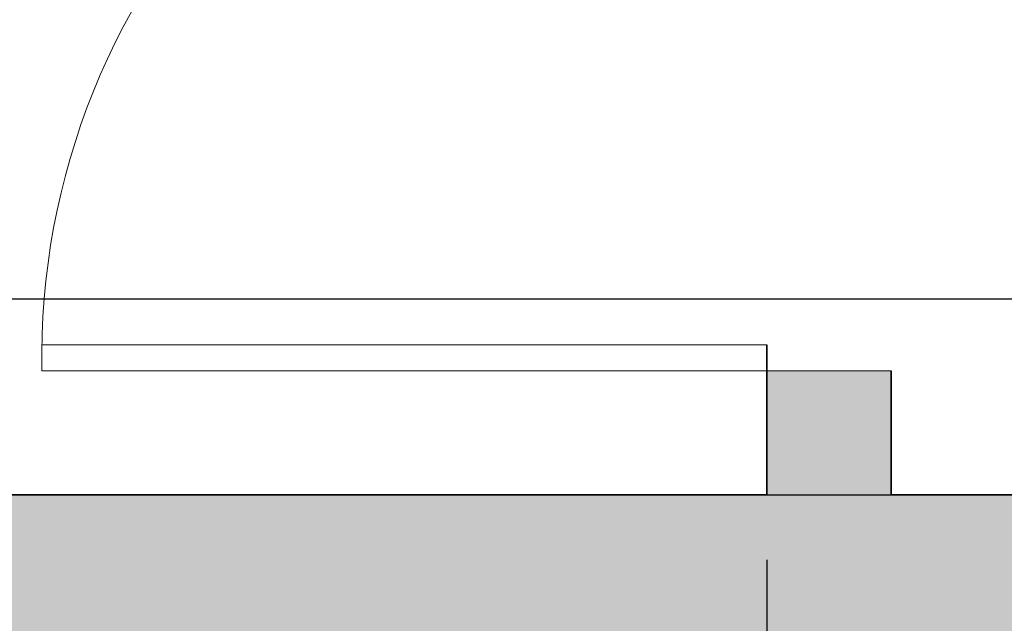
# Model space of a CAD drawing. Units: metres. Extents: x 4298.5 to 4325.2, y 2075 to 2095.8.
# Tile 10 of 35: x 4306.6693 to 4307.6197, y 2079.9341 to 2080.5171. Entities that reach past the tile are written whole.
import ezdxf

# ---------------------------------------------------------------- set-up
doc = ezdxf.new("R2010")
doc.units = ezdxf.units.M
for name, color, linetype, lineweight in [('A-ANNO-DIMS', 2, 'Continuous', 18), ('A-DOOR', 3, 'Continuous', 18), ('A-WALL', 7, 'Continuous', 35), ('A-WALL-PATT', 252, 'Continuous', 13)]:
    doc.layers.add(name, color=color, linetype=linetype, lineweight=lineweight)
doc.styles.get("Standard").update_dxf_attribs({"font": 'arial.ttf'})
doc.dimstyles.get("Standard").update_dxf_attribs({"dimtxt": 0.18, "dimasz": 0.18, "dimexe": 0.18, "dimexo": 0.0625, "dimgap": 0.09, "dimtad": 0, "dimtih": 1, "dimtoh": 1, "dimdec": 4, "dimzin": 0, "dimdsep": 46, "dimtxsty": 'Standard', "dimcen": 0.09, "dimadec": 0, "dimazin": 0, "dimtfac": 1, "dimtdec": 4, "dimtofl": 0, "dimtmove": 0, "dimatfit": 3, "dimfxl": 1, "dimtolj": 1, "dimtzin": 0, "dimarcsym": 0})

# ---------------------------------------------------------------- blocks, each defined once
blk = doc.blocks.new('DOOR-700-LEAF')
for p, q in [((0.67503, 0), (0.67503, 0.7)), ((0.70003, 0), (0.70003, 0.7))]:
    blk.add_line(p, q)
blk.add_arc((0.68753, 0.0125), 0.68761, 88.95837, 181.04163)
blk = doc.blocks.new('*D23')
at = {"layer": 'A-ANNO-DIMS', "color": 0, "lineweight": -2, "transparency": 16777216}
for p, q in [((4308.16058, 2079.85556), (4308.16058, 2079.58806)), ((4309.16058, 2079.85556), (4309.16058, 2079.58806)), ((4308.16058, 2079.76806), (4307.98058, 2079.76806)), ((4308.98058, 2079.76806), (4308.34058, 2079.76806))]:
    blk.add_line(p, q, dxfattribs=at)
at = {"layer": 'A-ANNO-DIMS', "color": 0, "transparency": 16777216}
for points in [[(4308.34058, 2079.79806), (4308.34058, 2079.73806), (4308.16058, 2079.76806)], [(4308.98058, 2079.79806), (4308.98058, 2079.73806), (4309.16058, 2079.76806)]]:
    blk.add_solid(points, dxfattribs=at)
at = {"layer": 'Defpoints', "color": 0, "transparency": 16777216}
for p in [(4308.16058, 2079.91806), (4309.16058, 2079.91806), (4308.16058, 2079.76806)]:
    blk.add_point(p, dxfattribs=at)
at = {"layer": 'A-ANNO-DIMS', "color": 0, "transparency": 16777216, "insert": (4306.70861, 2079.76806), "char_height": 0.18, "attachment_point": 5}
blk.add_mtext('\\A1;WINDOW W1 1 TYP.', dxfattribs=at)
blk = doc.blocks.new('*D47')
at = {"layer": 'A-ANNO-DIMS', "color": 0, "lineweight": -2, "transparency": 16777216}
for p, q in [((4300.43058, 2084.49556), (4300.43058, 2074.98956)), ((4322.81058, 2084.49556), (4322.81058, 2074.98956)), ((4300.61058, 2075.16956), (4311.22515, 2075.16956)), ((4322.63058, 2075.16956), (4312.016, 2075.16956))]:
    blk.add_line(p, q, dxfattribs=at)
at = {"layer": 'A-ANNO-DIMS', "color": 0, "transparency": 16777216}
for points in [[(4300.61058, 2075.19956), (4300.61058, 2075.13956), (4300.43058, 2075.16956)], [(4322.63058, 2075.19956), (4322.63058, 2075.13956), (4322.81058, 2075.16956)]]:
    blk.add_solid(points, dxfattribs=at)
at = {"layer": 'Defpoints', "color": 0, "transparency": 16777216}
for p in [(4300.43058, 2084.55806), (4322.81058, 2084.55806), (4322.81058, 2075.16956)]:
    blk.add_point(p, dxfattribs=at)
at = {"layer": 'A-ANNO-DIMS', "color": 0, "transparency": 16777216, "insert": (4311.62058, 2075.16956), "char_height": 0.18, "attachment_point": 5}
blk.add_mtext('\\A1;22.38', dxfattribs=at)
blk = doc.blocks.new('*D59')
at = {"layer": 'A-ANNO-DIMS', "color": 0, "lineweight": -2, "transparency": 16777216}
for p, q in [((4305.89058, 2079.99556), (4305.89058, 2074.98956)), ((4307.39058, 2079.99556), (4307.39058, 2074.98956)), ((4306.07058, 2075.16956), (4306.39452, 2075.16956)), ((4307.21058, 2075.16956), (4306.88663, 2075.16956))]:
    blk.add_line(p, q, dxfattribs=at)
at = {"layer": 'A-ANNO-DIMS', "color": 0, "transparency": 16777216}
for points in [[(4306.07058, 2075.19956), (4306.07058, 2075.13956), (4305.89058, 2075.16956)], [(4307.21058, 2075.19956), (4307.21058, 2075.13956), (4307.39058, 2075.16956)]]:
    blk.add_solid(points, dxfattribs=at)
at = {"layer": 'Defpoints', "color": 0, "transparency": 16777216}
for p in [(4305.89058, 2080.05806), (4307.39058, 2080.05806), (4307.39058, 2075.16956)]:
    blk.add_point(p, dxfattribs=at)
at = {"layer": 'A-ANNO-DIMS', "color": 0, "transparency": 16777216, "insert": (4306.64058, 2075.16956), "char_height": 0.18, "attachment_point": 5}
blk.add_mtext('\\A1;1.5', dxfattribs=at)
blk = doc.blocks.new('*D60')
at = {"layer": 'A-ANNO-DIMS', "color": 0, "lineweight": -2, "transparency": 16777216}
for p, q in [((4305.95308, 2081.93806), (4324.76712, 2081.93806)), ((4324.58712, 2081.75806), (4324.58712, 2081.17996)), ((4324.58712, 2080.23806), (4324.58712, 2080.81615)), ((4305.95308, 2080.05806), (4324.76712, 2080.05806))]:
    blk.add_line(p, q, dxfattribs=at)
at = {"layer": 'A-ANNO-DIMS', "color": 0, "transparency": 16777216}
for points in [[(4324.55712, 2081.75806), (4324.61712, 2081.75806), (4324.58712, 2081.93806)], [(4324.55712, 2080.23806), (4324.61712, 2080.23806), (4324.58712, 2080.05806)]]:
    blk.add_solid(points, dxfattribs=at)
at = {"layer": 'Defpoints', "color": 0, "transparency": 16777216}
for p in [(4305.89058, 2081.93806), (4324.58712, 2081.93806), (4305.89058, 2080.05806)]:
    blk.add_point(p, dxfattribs=at)
at = {"layer": 'A-ANNO-DIMS', "color": 0, "transparency": 16777216, "insert": (4324.58712, 2080.99806), "char_height": 0.18, "attachment_point": 5}
blk.add_mtext('\\A1;1.88', dxfattribs=at)
blk = doc.blocks.new('*D64')
at = {"layer": 'A-ANNO-DIMS', "color": 0, "lineweight": -2, "transparency": 16777216}
for p, q in [((4312.1097, 2081.12214), (4299.09208, 2081.12214)), ((4299.27208, 2080.94214), (4299.27208, 2080.42704)), ((4312.1097, 2080.24704), (4299.09208, 2080.24704)), ((4299.27208, 2080.24704), (4299.27208, 2080.06704)), ((4299.27208, 2080.06704), (4299.09208, 2080.06704))]:
    blk.add_line(p, q, dxfattribs=at)
at = {"layer": 'A-ANNO-DIMS', "color": 0, "transparency": 16777216}
for points in [[(4299.24208, 2080.94214), (4299.30208, 2080.94214), (4299.27208, 2081.12214)], [(4299.24208, 2080.42704), (4299.30208, 2080.42704), (4299.27208, 2080.24704)]]:
    blk.add_solid(points, dxfattribs=at)
at = {"layer": 'Defpoints', "color": 0, "transparency": 16777216}
for p in [(4312.1722, 2081.12214), (4299.27208, 2080.24704), (4312.1722, 2080.24704)]:
    blk.add_point(p, dxfattribs=at)
at = {"layer": 'A-ANNO-DIMS', "color": 0, "transparency": 16777216, "insert": (4298.76811, 2080.06704), "char_height": 0.18, "attachment_point": 5}
blk.add_mtext('\\A1;0.88', dxfattribs=at)

msp = doc.modelspace()

# ---------------------------------------------------------------- hatches: boundary and pattern name
at = {"layer": 'A-WALL-PATT'}
h = msp.add_hatch(color=256, dxfattribs=at)
h.dxf.hatch_style = 1
h.paths.add_polyline_path([(4308.76058, 2094.47806), (4308.16058, 2094.47806), (4307.46058, 2094.47806), (4307.46058, 2094.24806), (4308.27058, 2094.24806), (4308.27058, 2094.12806), (4308.39058, 2094.12806), (4308.39058, 2094.24806), (4308.76058, 2094.24806)])
h.paths.add_polyline_path([(4310.12058, 2094.47806), (4309.52058, 2094.47806), (4309.52058, 2094.24806), (4309.89058, 2094.24806), (4309.89058, 2092.24806), (4308.39058, 2092.24806), (4308.39058, 2093.42806), (4308.27058, 2093.42806), (4308.27058, 2092.01806), (4309.89058, 2092.01806), (4309.89058, 2087.01806), (4309.77058, 2087.01806), (4309.77058, 2086.78806), (4309.89058, 2086.78806), (4311.94058, 2086.78806), (4311.94058, 2087.01806), (4310.12058, 2087.01806), (4310.12058, 2089.01806), (4310.24058, 2089.01806), (4310.24058, 2089.13806), (4310.12058, 2089.13806), (4310.12058, 2092.01806), (4310.30785, 2092.01806), (4310.30785, 2092.24806), (4310.12058, 2092.24806)])
h.paths.add_polyline_path([(4311.74058, 2092.24806), (4311.06785, 2092.24806), (4311.06785, 2092.01806), (4311.74058, 2092.01806)], flags=17)
h.paths.add_polyline_path([(4313.17331, 2092.24806), (4312.50058, 2092.24806), (4312.50058, 2092.01806), (4313.17331, 2092.01806)])
h.paths.add_polyline_path([(4314.53785, 2092.24806), (4314.12058, 2092.24806), (4313.93331, 2092.24806), (4313.93331, 2092.01806), (4314.12058, 2092.01806), (4314.12058, 2087.01806), (4314.00058, 2087.01806), (4314.00058, 2086.78806), (4314.12058, 2086.78806), (4315.57179, 2086.78806), (4315.57179, 2087.01806), (4314.35058, 2087.01806), (4314.35058, 2092.01806), (4314.53785, 2092.01806)])
h.paths.add_polyline_path([(4315.97058, 2092.24806), (4315.29785, 2092.24806), (4315.29785, 2092.01806), (4315.97058, 2092.01806)])
h.paths.add_polyline_path([(4317.40331, 2092.24806), (4316.73058, 2092.24806), (4316.73058, 2092.01806), (4317.40331, 2092.01806)])
h.paths.add_polyline_path([(4318.95058, 2092.24806), (4318.35058, 2092.24806), (4318.16331, 2092.24806), (4318.16331, 2092.01806), (4318.35058, 2092.01806), (4318.35058, 2091.89806), (4318.58058, 2091.89806), (4318.58058, 2092.01806), (4318.95058, 2092.01806)])
h.paths.add_polyline_path([(4321.01058, 2092.24806), (4319.71058, 2092.24806), (4319.71058, 2092.01806), (4320.08058, 2092.01806), (4320.08058, 2090.01806), (4318.58058, 2090.01806), (4318.58058, 2091.19806), (4318.35058, 2091.19806), (4318.35058, 2090.01806), (4318.35058, 2087.01806), (4318.23058, 2087.01806), (4318.23058, 2086.78806), (4318.35058, 2086.78806), (4318.35058, 2086.30806), (4318.58058, 2086.30806), (4318.58058, 2089.78806), (4321.78058, 2089.78806), (4321.78058, 2090.01806), (4320.20058, 2090.01806), (4320.20058, 2092.01806), (4321.01058, 2092.01806)])
h.paths.add_polyline_path([(4322.81058, 2092.24806), (4321.77058, 2092.24806), (4321.77058, 2092.01806), (4322.58058, 2092.01806), (4322.58058, 2091.28306), (4322.81058, 2091.28306)])
h.paths.add_polyline_path([(4322.81058, 2090.52306), (4322.58058, 2090.52306), (4322.58058, 2089.78806), (4322.58058, 2089.52545), (4322.81058, 2089.52545), (4322.81058, 2090.01806)])
h.paths.add_polyline_path([(4322.81058, 2088.76545), (4322.58058, 2088.76545), (4322.58058, 2087.66806), (4322.81058, 2087.66806)])
h.paths.add_polyline_path([(4322.81058, 2086.90806), (4322.58058, 2086.90806), (4322.58058, 2085.81066), (4322.81058, 2085.81066)])
h.paths.add_polyline_path([(4322.81058, 2085.05066), (4322.58058, 2085.05066), (4322.58058, 2084.78806), (4318.58058, 2084.78806), (4318.58058, 2085.05806), (4318.58058, 2085.40806), (4318.35058, 2085.40806), (4318.35058, 2084.55806), (4318.35058, 2080.85806), (4318.47058, 2080.85806), (4318.47058, 2082.32806), (4319.26058, 2082.32806), (4319.26058, 2082.55806), (4318.58058, 2082.55806), (4318.58058, 2084.55806), (4320.08058, 2084.55806), (4320.08058, 2083.93806), (4320.31058, 2083.93806), (4320.31058, 2084.55806), (4322.81058, 2084.55806)])
h.paths.add_polyline_path([(4320.31058, 2083.17806), (4320.08058, 2083.17806), (4320.08058, 2082.55806), (4319.96058, 2082.55806), (4319.96058, 2082.32806), (4320.08058, 2082.32806), (4320.08058, 2081.57306), (4320.31058, 2081.57306)], flags=17)
h.paths.add_polyline_path([(4320.31058, 2080.81306), (4320.08058, 2080.81306), (4320.08058, 2080.05806), (4318.42861, 2080.05806), (4318.42861, 2079.82806), (4320.31058, 2079.82806)])
h.paths.add_polyline_path([(4317.35058, 2085.28806), (4316.57179, 2085.28806), (4316.57179, 2085.05806), (4317.35058, 2085.05806)])
h.paths.add_polyline_path([(4315.57179, 2085.28806), (4314.84342, 2085.28806), (4314.84342, 2085.05806), (4315.57179, 2085.05806)])
h.paths.add_polyline_path([(4313.84342, 2085.28806), (4312.94058, 2085.28806), (4312.94058, 2085.05806), (4313.84342, 2085.05806)])
h.paths.add_polyline_path([(4311.94058, 2085.28806), (4311.44058, 2085.28806), (4311.44058, 2085.05806), (4311.94058, 2085.05806)])
h.paths.add_polyline_path([(4317.33058, 2087.01806), (4316.57179, 2087.01806), (4316.57179, 2086.78806), (4317.33058, 2086.78806)])
h.paths.add_polyline_path([(4313.10058, 2089.13806), (4311.14058, 2089.13806), (4311.14058, 2089.01806), (4312.98058, 2089.01806), (4312.98058, 2087.01806), (4312.94058, 2087.01806), (4312.94058, 2086.78806), (4313.10058, 2086.78806), (4313.10058, 2087.01806)])
h.paths.add_polyline_path([(4307.55152, 2087.01806), (4305.89058, 2087.01806), (4305.89058, 2092.24806), (4305.89058, 2094.24806), (4306.70058, 2094.24806), (4306.70058, 2094.47806), (4305.66058, 2094.47806), (4305.66058, 2092.24806), (4305.29058, 2092.24806), (4305.29058, 2092.01806), (4305.66058, 2092.01806), (4305.66058, 2090.01806), (4304.16058, 2090.01806), (4304.16058, 2091.19806), (4304.04058, 2091.19806), (4304.04058, 2089.90806), (4301.56058, 2089.90806), (4301.56058, 2089.78806), (4304.04058, 2089.78806), (4305.66058, 2089.78806), (4305.66058, 2086.63806), (4305.89058, 2086.63806), (4305.89058, 2086.78806), (4307.55152, 2086.78806)])
h.paths.add_polyline_path([(4307.55152, 2085.28806), (4305.89058, 2085.28806), (4305.89058, 2085.43806), (4305.66058, 2085.43806), (4305.66058, 2084.78806), (4305.29058, 2084.78806), (4305.29058, 2084.55806), (4305.66058, 2084.55806), (4305.66058, 2084.02001), (4305.89058, 2084.02001), (4305.89058, 2084.55806), (4305.89058, 2085.05806), (4307.55152, 2085.05806)])
h.paths.add_polyline_path([(4310.24058, 2085.28806), (4308.55152, 2085.28806), (4308.55152, 2085.05806), (4310.24058, 2085.05806)])
h.paths.add_polyline_path([(4317.42861, 2080.05806), (4316.57179, 2080.05806), (4316.57179, 2079.82806), (4317.42861, 2079.82806)])
h.paths.add_polyline_path([(4315.57179, 2080.05806), (4314.84342, 2080.05806), (4314.84342, 2079.82806), (4315.57179, 2079.82806)])
h.paths.add_polyline_path([(4313.84342, 2080.05806), (4312.94058, 2080.05806), (4312.94058, 2079.82806), (4313.84342, 2079.82806)])
h.paths.add_polyline_path([(4311.94058, 2080.05806), (4311.44058, 2080.05806), (4311.44058, 2079.82806), (4311.94058, 2079.82806)])
h.paths.add_polyline_path([(4310.24058, 2080.05806), (4310.12058, 2080.05806), (4310.12058, 2084.03806), (4309.89058, 2084.03806), (4309.89058, 2080.05806), (4309.16058, 2080.05806), (4309.16058, 2079.82806), (4310.24058, 2079.82806)])
h.paths.add_polyline_path([(4308.16058, 2080.05806), (4307.51058, 2080.05806), (4307.51058, 2080.17806), (4307.39058, 2080.17806), (4307.39058, 2080.05806), (4305.89058, 2080.05806), (4305.89058, 2080.56697), (4305.66058, 2080.56697), (4305.66058, 2079.82806), (4308.16058, 2079.82806)])
h.paths.add_polyline_path([(4307.51058, 2081.93806), (4309.09058, 2081.93806), (4309.09058, 2082.05806), (4305.89058, 2082.05806), (4305.89058, 2083.26001), (4305.66058, 2083.26001), (4305.66058, 2081.32697), (4305.89058, 2081.32697), (4305.89058, 2081.93806), (4307.39058, 2081.93806), (4307.39058, 2080.87806), (4307.51058, 2080.87806)])
h.paths.add_polyline_path([(4304.53058, 2084.78806), (4302.73058, 2084.78806), (4302.73058, 2084.55806), (4304.53058, 2084.55806)])
h.paths.add_polyline_path([(4301.97058, 2084.78806), (4300.66058, 2084.78806), (4300.66058, 2085.02492), (4300.43058, 2085.02492), (4300.43058, 2084.55806), (4301.97058, 2084.55806)])
h.paths.add_polyline_path([(4300.66058, 2086.88429), (4300.43058, 2086.88429), (4300.43058, 2085.78492), (4300.66058, 2085.78492)])
h.paths.add_polyline_path([(4300.66058, 2089.16182), (4300.43058, 2089.16182), (4300.43058, 2087.64429), (4300.66058, 2087.64429)])
h.paths.add_polyline_path([(4300.66058, 2091.02119), (4300.43058, 2091.02119), (4300.43058, 2089.92182), (4300.66058, 2089.92182)])
h.paths.add_polyline_path([(4300.66058, 2092.01806), (4301.97058, 2092.01806), (4301.97058, 2092.24806), (4300.43058, 2092.24806), (4300.43058, 2091.78119), (4300.66058, 2091.78119)])
h.paths.add_polyline_path([(4304.53058, 2092.24806), (4302.73058, 2092.24806), (4302.73058, 2092.01806), (4304.04058, 2092.01806), (4304.04058, 2091.89806), (4304.16058, 2091.89806), (4304.16058, 2092.01806), (4304.53058, 2092.01806)], flags=17)

# ---------------------------------------------------------------- linework, layer by layer
at = {"layer": 'A-DOOR'}
msp.add_line((4307.39058, 2080.17806), (4307.51058, 2080.17806), dxfattribs=at)
at = {"layer": 'A-WALL'}
for p, q in [((4307.39058, 2080.20306), (4307.39058, 2080.05806)), ((4307.51058, 2080.17806), (4307.51058, 2080.05806)), ((4305.89058, 2080.05806), (4307.39058, 2080.05806)), ((4307.51058, 2080.05806), (4309.89058, 2080.05806))]:
    msp.add_line(p, q, dxfattribs=at)

# ---------------------------------------------------------------- block references
at = {"layer": 'A-DOOR', "extrusion": (0, 0, -1), "zscale": -1, "rotation": 270.0000000000699}
msp.add_blockref('DOOR-700-LEAF', (-4307.39058, 2080.87808), dxfattribs=at)

# ---------------------------------------------------------------- dimensions: what is measured, and where the dimension line sits
at = {"layer": 'A-ANNO-DIMS'}
for base, p1, p2, override, picture, middle in [((4322.81058, 2075.16956), (4300.43058, 2084.55806), (4322.81058, 2084.55806), {"dimdec": 2, "dimlfac": 1, "dimrnd": 0, "dimzin": 0, "dimdsep": 46, "dimlunit": 2}, '*D47', (4311.62058, 2075.16956)), ((4307.39058, 2075.16956), (4305.89058, 2080.05806), (4307.39058, 2080.05806), {"dimdec": 1, "dimlfac": 1, "dimrnd": 0, "dimzin": 0, "dimdsep": 46, "dimlunit": 2}, '*D59', (4306.64058, 2075.16956))]:
    dim = msp.add_linear_dim(base=base, p1=p1, p2=p2, dimstyle='Standard', override=override, dxfattribs=at)
    dim.commit()
    dim.dimension.update_dxf_attribs({"geometry": picture, "text_midpoint": middle})
for base, p1, p2, picture, middle in [((4324.58712, 2081.93806), (4305.89058, 2080.05806), (4305.89058, 2081.93806), '*D60', (4324.58712, 2080.99806)), ((4299.27208, 2080.24704), (4312.1722, 2081.12214), (4312.1722, 2080.24704), '*D64', (4298.76811, 2080.06704))]:
    dim = msp.add_linear_dim(base=base, p1=p1, p2=p2, angle=90, dimstyle='Standard', override={"dimdec": 2, "dimlfac": 1, "dimrnd": 0, "dimzin": 0, "dimdsep": 46, "dimlunit": 2}, dxfattribs=at)
    dim.commit()
    dim.dimension.update_dxf_attribs({"geometry": picture, "text_midpoint": middle})
dim = msp.add_linear_dim(base=(4308.16058, 2079.76806), p1=(4309.16058, 2079.91806), p2=(4308.16058, 2079.91806), angle=180, text='WINDOW W1 <> TYP.', dimstyle='Standard', override={"dimdec": 0, "dimlfac": 1, "dimrnd": 0, "dimzin": 0, "dimdsep": 46, "dimlunit": 2}, dxfattribs=at)
dim.commit()
dim.dimension.update_dxf_attribs({"geometry": '*D23', "text_midpoint": (4306.70861, 2079.76806)})

doc.saveas('drawing.dxf')
